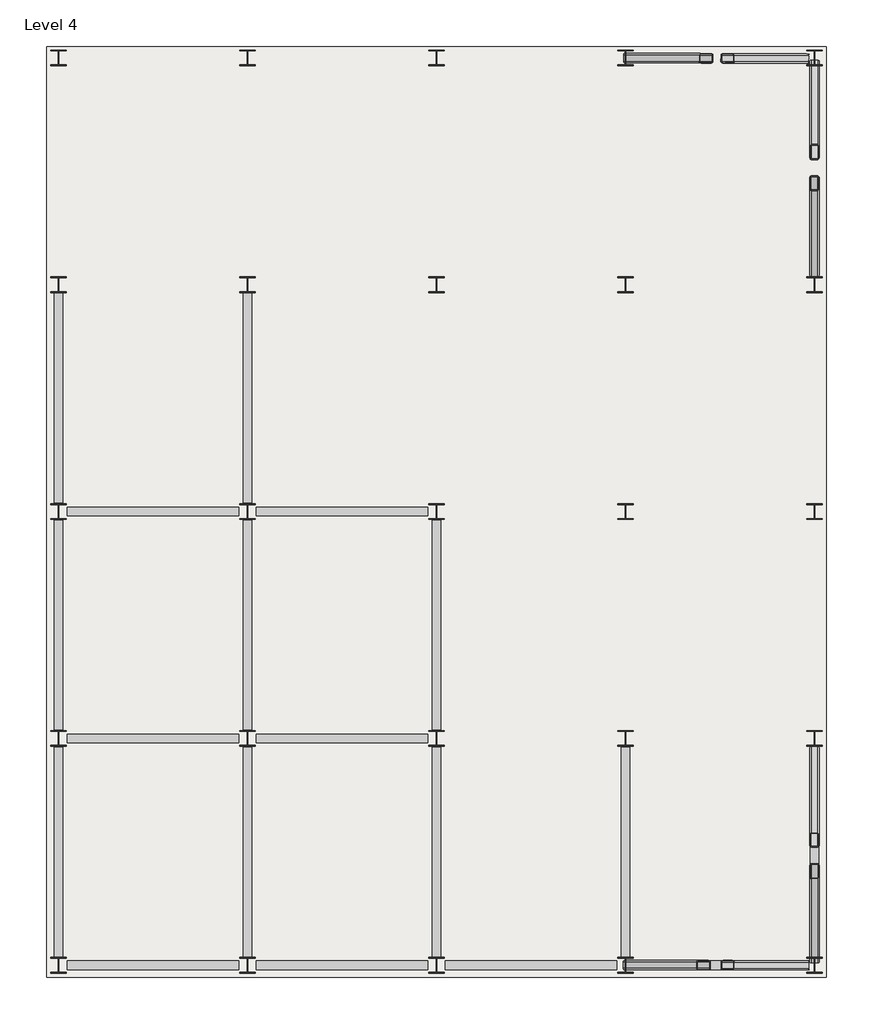
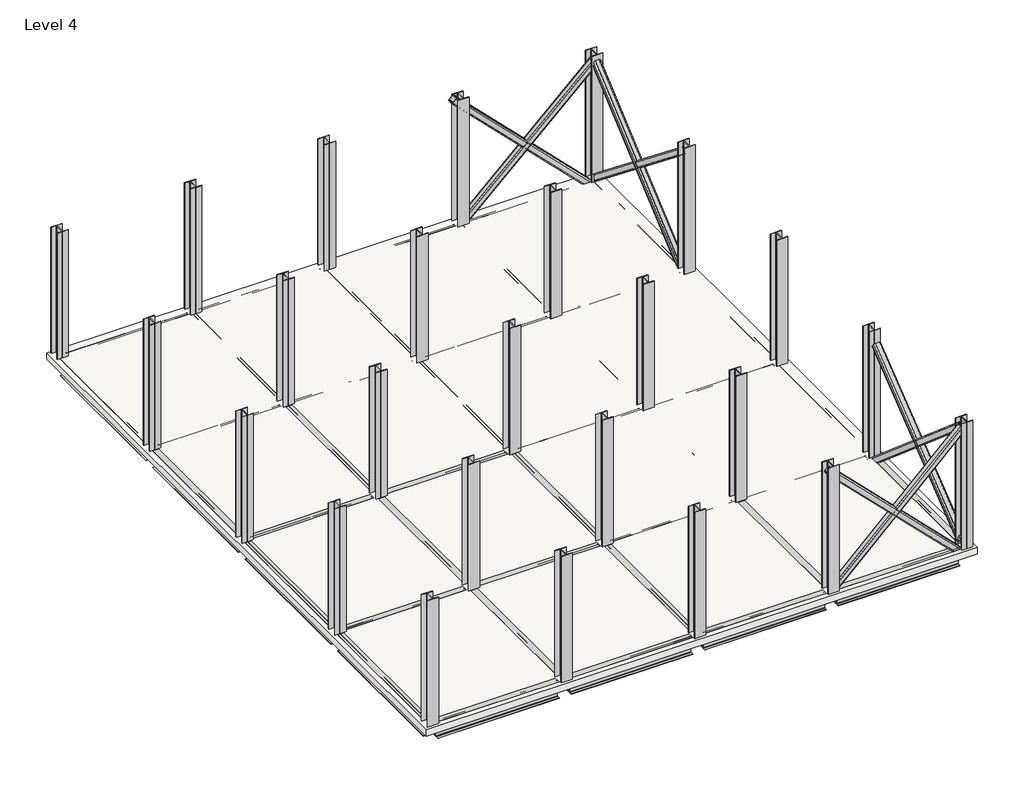
# One storey: 40 beams, 25 columns, 8 members, 1 slab.
"""IFC4 building model written with IfcOpenShell, lengths in millimetres."""

from ifc_helpers import new_model, si_unit, frame, origin, place, context, project, spatial, polyline, outline, extrude, transform, mapped, element, save
from components import w_shapes_w16x26_71b85d0e, w_shapes_w16x26_5730d789, w_shapes_column_w10x49_8035b166, hss_square_hss6x6x1_2_008024fe, hss_square_hss6x6x1_2_7c43692b, hss_square_hss6x6x1_2_5f011b37, hss_square_hss6x6x1_2_b9926e2d, hss_square_hss6x6x1_2_e6555cf9, hss_square_hss6x6x1_2_f7a49a43, hss_square_hss6x6x1_2_10b7330d, hss_square_hss6x6x1_2_f3b36863

model = new_model("IFC4")

# Units and contexts
model_context = context("Model", 3, world=origin())
ifc_project = project(units=[si_unit("LENGTHUNIT", "METRE", prefix="MILLI")], contexts=[model_context])

# Site, building, storey
site = spatial("IfcSite", under=ifc_project)
building = spatial("IfcBuilding", under=site)
storey = spatial("IfcBuildingStorey", under=building, Name="Level 4", Elevation=9144.0)

# Beams
placement = place(None, origin())
w_shapes_w16x26_shape = w_shapes_w16x26_71b85d0e(model_context)
element("IfcBeam", 1, ObjectType="W Shapes : W16X26", at=placement, inside=storey, context=model_context, shape_type="MappedRepresentation", body=[
    mapped(w_shapes_w16x26_shape, transform((-5883.5186598, -2213.7239423, 8944.61), x_axis=(1.0, 0.0, 0.0), y_axis=(0.0, 1.0, 0.0), z_axis=(0.0, 0.0, 1.0))),
])
element("IfcBeam", 2, ObjectType="W Shapes : W16X26", at=placement, inside=storey, context=model_context, shape_type="MappedRepresentation", body=[
    mapped(w_shapes_w16x26_shape, transform((-2835.5186598, -2213.7239423, 8944.61), x_axis=(1.0, 0.0, 0.0), y_axis=(0.0, 1.0, 0.0), z_axis=(0.0, 0.0, 1.0))),
])
element("IfcBeam", 3, ObjectType="W Shapes : W16X26", at=placement, inside=storey, context=model_context, shape_type="MappedRepresentation", body=[
    mapped(w_shapes_w16x26_shape, transform((212.4813402, -2213.7239423, 8944.61), x_axis=(1.0, 0.0, 0.0), y_axis=(0.0, 1.0, 0.0), z_axis=(0.0, 0.0, 1.0))),
])
element("IfcBeam", 4, ObjectType="W Shapes : W16X26", at=placement, inside=storey, context=model_context, shape_type="MappedRepresentation", body=[
    mapped(w_shapes_w16x26_shape, transform((3260.4813402, -2213.7239423, 8944.61), x_axis=(1.0, 0.0, 0.0), y_axis=(0.0, 1.0, 0.0), z_axis=(0.0, 0.0, 1.0))),
])
element("IfcBeam", 5, ObjectType="W Shapes : W16X26", at=placement, inside=storey, context=model_context, shape_type="MappedRepresentation", body=[
    mapped(w_shapes_w16x26_shape, transform((-5883.5186598, 1443.8760577, 8944.61), x_axis=(1.0, 0.0, 0.0), y_axis=(0.0, 1.0, 0.0), z_axis=(0.0, 0.0, 1.0))),
])
element("IfcBeam", 6, ObjectType="W Shapes : W16X26", at=placement, inside=storey, context=model_context, shape_type="MappedRepresentation", body=[
    mapped(w_shapes_w16x26_shape, transform((-2835.5186598, 1443.8760577, 8944.61), x_axis=(1.0, 0.0, 0.0), y_axis=(0.0, 1.0, 0.0), z_axis=(0.0, 0.0, 1.0))),
])
element("IfcBeam", 7, ObjectType="W Shapes : W16X26", at=placement, inside=storey, context=model_context, shape_type="MappedRepresentation", body=[
    mapped(w_shapes_w16x26_shape, transform((212.4813402, 1443.8760577, 8944.61), x_axis=(1.0, 0.0, 0.0), y_axis=(0.0, 1.0, 0.0), z_axis=(0.0, 0.0, 1.0))),
])
element("IfcBeam", 8, ObjectType="W Shapes : W16X26", at=placement, inside=storey, context=model_context, shape_type="MappedRepresentation", body=[
    mapped(w_shapes_w16x26_shape, transform((3260.4813402, 1443.8760577, 8944.61), x_axis=(1.0, 0.0, 0.0), y_axis=(0.0, 1.0, 0.0), z_axis=(0.0, 0.0, 1.0))),
])
element("IfcBeam", 9, ObjectType="W Shapes : W16X26", at=placement, inside=storey, context=model_context, shape_type="MappedRepresentation", body=[
    mapped(w_shapes_w16x26_shape, transform((-5883.5186598, 5101.4760577, 8944.61), x_axis=(1.0, 0.0, 0.0), y_axis=(0.0, 1.0, 0.0), z_axis=(0.0, 0.0, 1.0))),
])
element("IfcBeam", 10, ObjectType="W Shapes : W16X26", at=placement, inside=storey, context=model_context, shape_type="MappedRepresentation", body=[
    mapped(w_shapes_w16x26_shape, transform((-2835.5186598, 5101.4760577, 8944.61), x_axis=(1.0, 0.0, 0.0), y_axis=(0.0, 1.0, 0.0), z_axis=(0.0, 0.0, 1.0))),
])
element("IfcBeam", 11, ObjectType="W Shapes : W16X26", at=placement, inside=storey, context=model_context, shape_type="MappedRepresentation", body=[
    mapped(w_shapes_w16x26_shape, transform((212.4813402, 5101.4760577, 8944.61), x_axis=(1.0, 0.0, 0.0), y_axis=(0.0, 1.0, 0.0), z_axis=(0.0, 0.0, 1.0))),
])
element("IfcBeam", 12, ObjectType="W Shapes : W16X26", at=placement, inside=storey, context=model_context, shape_type="MappedRepresentation", body=[
    mapped(w_shapes_w16x26_shape, transform((3260.4813402, 5101.4760577, 8944.61), x_axis=(1.0, 0.0, 0.0), y_axis=(0.0, 1.0, 0.0), z_axis=(0.0, 0.0, 1.0))),
])
element("IfcBeam", 13, ObjectType="W Shapes : W16X26", at=placement, inside=storey, context=model_context, shape_type="MappedRepresentation", body=[
    mapped(w_shapes_w16x26_shape, transform((-5883.5186598, 8759.0760577, 8944.61), x_axis=(1.0, 0.0, 0.0), y_axis=(0.0, 1.0, 0.0), z_axis=(0.0, 0.0, 1.0))),
])
element("IfcBeam", 14, ObjectType="W Shapes : W16X26", at=placement, inside=storey, context=model_context, shape_type="MappedRepresentation", body=[
    mapped(w_shapes_w16x26_shape, transform((-2835.5186598, 8759.0760577, 8944.61), x_axis=(1.0, 0.0, 0.0), y_axis=(0.0, 1.0, 0.0), z_axis=(0.0, 0.0, 1.0))),
])
element("IfcBeam", 15, ObjectType="W Shapes : W16X26", at=placement, inside=storey, context=model_context, shape_type="MappedRepresentation", body=[
    mapped(w_shapes_w16x26_shape, transform((212.4813402, 8759.0760577, 8944.61), x_axis=(1.0, 0.0, 0.0), y_axis=(0.0, 1.0, 0.0), z_axis=(0.0, 0.0, 1.0))),
])
element("IfcBeam", 16, ObjectType="W Shapes : W16X26", at=placement, inside=storey, context=model_context, shape_type="MappedRepresentation", body=[
    mapped(w_shapes_w16x26_shape, transform((3260.4813402, 8759.0760577, 8944.61), x_axis=(1.0, 0.0, 0.0), y_axis=(0.0, 1.0, 0.0), z_axis=(0.0, 0.0, 1.0))),
])
element("IfcBeam", 17, ObjectType="W Shapes : W16X26", at=placement, inside=storey, context=model_context, shape_type="MappedRepresentation", body=[
    mapped(w_shapes_w16x26_shape, transform((-5883.5186598, 12416.6760577, 8944.61), x_axis=(1.0, 0.0, 0.0), y_axis=(0.0, 1.0, 0.0), z_axis=(0.0, 0.0, 1.0))),
])
element("IfcBeam", 18, ObjectType="W Shapes : W16X26", at=placement, inside=storey, context=model_context, shape_type="MappedRepresentation", body=[
    mapped(w_shapes_w16x26_shape, transform((-2835.5186598, 12416.6760577, 8944.61), x_axis=(1.0, 0.0, 0.0), y_axis=(0.0, 1.0, 0.0), z_axis=(0.0, 0.0, 1.0))),
])
element("IfcBeam", 19, ObjectType="W Shapes : W16X26", at=placement, inside=storey, context=model_context, shape_type="MappedRepresentation", body=[
    mapped(w_shapes_w16x26_shape, transform((212.4813402, 12416.6760577, 8944.61), x_axis=(1.0, 0.0, 0.0), y_axis=(0.0, 1.0, 0.0), z_axis=(0.0, 0.0, 1.0))),
])
element("IfcBeam", 20, ObjectType="W Shapes : W16X26", at=placement, inside=storey, context=model_context, shape_type="MappedRepresentation", body=[
    mapped(w_shapes_w16x26_shape, transform((3260.4813402, 12416.6760577, 8944.61), x_axis=(1.0, 0.0, 0.0), y_axis=(0.0, 1.0, 0.0), z_axis=(0.0, 0.0, 1.0))),
])
w_shapes_w16x26_2_shape = w_shapes_w16x26_5730d789(model_context)
element("IfcBeam", 21, ObjectType="W Shapes : W16X26", at=placement, inside=storey, context=model_context, shape_type="MappedRepresentation", body=[
    mapped(w_shapes_w16x26_2_shape, transform((4784.4813402, 10587.8760577, 8944.61), x_axis=(0.0, -1.0, 0.0), y_axis=(1.0, 0.0, 0.0), z_axis=(0.0, 0.0, 1.0))),
])
element("IfcBeam", 22, ObjectType="W Shapes : W16X26", at=placement, inside=storey, context=model_context, shape_type="MappedRepresentation", body=[
    mapped(w_shapes_w16x26_2_shape, transform((4784.4813402, 6930.2760577, 8944.61), x_axis=(0.0, -1.0, 0.0), y_axis=(1.0, 0.0, 0.0), z_axis=(0.0, 0.0, 1.0))),
])
element("IfcBeam", 23, ObjectType="W Shapes : W16X26", at=placement, inside=storey, context=model_context, shape_type="MappedRepresentation", body=[
    mapped(w_shapes_w16x26_2_shape, transform((4784.4813402, 3272.6760577, 8944.61), x_axis=(0.0, -1.0, 0.0), y_axis=(1.0, 0.0, 0.0), z_axis=(0.0, 0.0, 1.0))),
])
element("IfcBeam", 24, ObjectType="W Shapes : W16X26", at=placement, inside=storey, context=model_context, shape_type="MappedRepresentation", body=[
    mapped(w_shapes_w16x26_2_shape, transform((4784.4813402, -384.9239423, 8944.61), x_axis=(0.0, -1.0, 0.0), y_axis=(1.0, 0.0, 0.0), z_axis=(0.0, 0.0, 1.0))),
])
element("IfcBeam", 25, ObjectType="W Shapes : W16X26", at=placement, inside=storey, context=model_context, shape_type="MappedRepresentation", body=[
    mapped(w_shapes_w16x26_2_shape, transform((1736.4813402, 10587.8760577, 8944.61), x_axis=(0.0, -1.0, 0.0), y_axis=(1.0, 0.0, 0.0), z_axis=(0.0, 0.0, 1.0))),
])
element("IfcBeam", 26, ObjectType="W Shapes : W16X26", at=placement, inside=storey, context=model_context, shape_type="MappedRepresentation", body=[
    mapped(w_shapes_w16x26_2_shape, transform((1736.4813402, 6930.2760577, 8944.61), x_axis=(0.0, -1.0, 0.0), y_axis=(1.0, 0.0, 0.0), z_axis=(0.0, 0.0, 1.0))),
])
element("IfcBeam", 27, ObjectType="W Shapes : W16X26", at=placement, inside=storey, context=model_context, shape_type="MappedRepresentation", body=[
    mapped(w_shapes_w16x26_2_shape, transform((1736.4813402, 3272.6760577, 8944.61), x_axis=(0.0, -1.0, 0.0), y_axis=(1.0, 0.0, 0.0), z_axis=(0.0, 0.0, 1.0))),
])
element("IfcBeam", 28, ObjectType="W Shapes : W16X26", at=placement, inside=storey, context=model_context, shape_type="MappedRepresentation", body=[
    mapped(w_shapes_w16x26_2_shape, transform((1736.4813402, -384.9239423, 8944.61), x_axis=(0.0, -1.0, 0.0), y_axis=(1.0, 0.0, 0.0), z_axis=(0.0, 0.0, 1.0))),
])
element("IfcBeam", 29, ObjectType="W Shapes : W16X26", at=placement, inside=storey, context=model_context, shape_type="MappedRepresentation", body=[
    mapped(w_shapes_w16x26_2_shape, transform((-1311.5186598, 10587.8760577, 8944.61), x_axis=(0.0, -1.0, 0.0), y_axis=(1.0, 0.0, 0.0), z_axis=(0.0, 0.0, 1.0))),
])
element("IfcBeam", 30, ObjectType="W Shapes : W16X26", at=placement, inside=storey, context=model_context, shape_type="MappedRepresentation", body=[
    mapped(w_shapes_w16x26_2_shape, transform((-1311.5186598, 6930.2760577, 8944.61), x_axis=(0.0, -1.0, 0.0), y_axis=(1.0, 0.0, 0.0), z_axis=(0.0, 0.0, 1.0))),
])
element("IfcBeam", 31, ObjectType="W Shapes : W16X26", at=placement, inside=storey, context=model_context, shape_type="MappedRepresentation", body=[
    mapped(w_shapes_w16x26_2_shape, transform((-1311.5186598, 3272.6760577, 8944.61), x_axis=(0.0, -1.0, 0.0), y_axis=(1.0, 0.0, 0.0), z_axis=(0.0, 0.0, 1.0))),
])
element("IfcBeam", 32, ObjectType="W Shapes : W16X26", at=placement, inside=storey, context=model_context, shape_type="MappedRepresentation", body=[
    mapped(w_shapes_w16x26_2_shape, transform((-1311.5186598, -384.9239423, 8944.61), x_axis=(0.0, -1.0, 0.0), y_axis=(1.0, 0.0, 0.0), z_axis=(0.0, 0.0, 1.0))),
])
element("IfcBeam", 33, ObjectType="W Shapes : W16X26", at=placement, inside=storey, context=model_context, shape_type="MappedRepresentation", body=[
    mapped(w_shapes_w16x26_2_shape, transform((-4359.5186598, 10587.8760577, 8944.61), x_axis=(0.0, -1.0, 0.0), y_axis=(1.0, 0.0, 0.0), z_axis=(0.0, 0.0, 1.0))),
])
element("IfcBeam", 34, ObjectType="W Shapes : W16X26", at=placement, inside=storey, context=model_context, shape_type="MappedRepresentation", body=[
    mapped(w_shapes_w16x26_2_shape, transform((-4359.5186598, 6930.2760577, 8944.61), x_axis=(0.0, -1.0, 0.0), y_axis=(1.0, 0.0, 0.0), z_axis=(0.0, 0.0, 1.0))),
])
element("IfcBeam", 35, ObjectType="W Shapes : W16X26", at=placement, inside=storey, context=model_context, shape_type="MappedRepresentation", body=[
    mapped(w_shapes_w16x26_2_shape, transform((-4359.5186598, 3272.6760577, 8944.61), x_axis=(0.0, -1.0, 0.0), y_axis=(1.0, 0.0, 0.0), z_axis=(0.0, 0.0, 1.0))),
])
element("IfcBeam", 36, ObjectType="W Shapes : W16X26", at=placement, inside=storey, context=model_context, shape_type="MappedRepresentation", body=[
    mapped(w_shapes_w16x26_2_shape, transform((-4359.5186598, -384.9239423, 8944.61), x_axis=(0.0, -1.0, 0.0), y_axis=(1.0, 0.0, 0.0), z_axis=(0.0, 0.0, 1.0))),
])
element("IfcBeam", 37, ObjectType="W Shapes : W16X26", at=placement, inside=storey, context=model_context, shape_type="MappedRepresentation", body=[
    mapped(w_shapes_w16x26_2_shape, transform((-7407.5186598, 10587.8760577, 8944.61), x_axis=(0.0, -1.0, 0.0), y_axis=(1.0, 0.0, 0.0), z_axis=(0.0, 0.0, 1.0))),
])
element("IfcBeam", 38, ObjectType="W Shapes : W16X26", at=placement, inside=storey, context=model_context, shape_type="MappedRepresentation", body=[
    mapped(w_shapes_w16x26_2_shape, transform((-7407.5186598, 6930.2760577, 8944.61), x_axis=(0.0, -1.0, 0.0), y_axis=(1.0, 0.0, 0.0), z_axis=(0.0, 0.0, 1.0))),
])
element("IfcBeam", 39, ObjectType="W Shapes : W16X26", at=placement, inside=storey, context=model_context, shape_type="MappedRepresentation", body=[
    mapped(w_shapes_w16x26_2_shape, transform((-7407.5186598, 3272.6760577, 8944.61), x_axis=(0.0, -1.0, 0.0), y_axis=(1.0, 0.0, 0.0), z_axis=(0.0, 0.0, 1.0))),
])
element("IfcBeam", 40, ObjectType="W Shapes : W16X26", at=placement, inside=storey, context=model_context, shape_type="MappedRepresentation", body=[
    mapped(w_shapes_w16x26_2_shape, transform((-7407.5186598, -384.9239423, 8944.61), x_axis=(0.0, -1.0, 0.0), y_axis=(1.0, 0.0, 0.0), z_axis=(0.0, 0.0, 1.0))),
])

# Columns
w_shapes_column_w10x49_shape = w_shapes_column_w10x49_8035b166(model_context)
element("IfcColumn", 41, ObjectType="W Shapes-Column : W10X49", at=placement, inside=storey, context=model_context, shape_type="MappedRepresentation", body=[
    mapped(w_shapes_column_w10x49_shape, transform((4784.4813402, -2213.7239423, 0.0), x_axis=(1.0, 0.0, 0.0), y_axis=(0.0, 1.0, 0.0), z_axis=(0.0, 0.0, 1.0))),
])
element("IfcColumn", 42, ObjectType="W Shapes-Column : W10X49", at=placement, inside=storey, context=model_context, shape_type="MappedRepresentation", body=[
    mapped(w_shapes_column_w10x49_shape, transform((1736.4813402, -2213.7239423, 0.0), x_axis=(1.0, 0.0, 0.0), y_axis=(0.0, 1.0, 0.0), z_axis=(0.0, 0.0, 1.0))),
])
element("IfcColumn", 43, ObjectType="W Shapes-Column : W10X49", at=placement, inside=storey, context=model_context, shape_type="MappedRepresentation", body=[
    mapped(w_shapes_column_w10x49_shape, transform((-1311.5186598, -2213.7239423, 0.0), x_axis=(1.0, 0.0, 0.0), y_axis=(0.0, 1.0, 0.0), z_axis=(0.0, 0.0, 1.0))),
])
element("IfcColumn", 44, ObjectType="W Shapes-Column : W10X49", at=placement, inside=storey, context=model_context, shape_type="MappedRepresentation", body=[
    mapped(w_shapes_column_w10x49_shape, transform((-4359.5186598, -2213.7239423, 0.0), x_axis=(1.0, 0.0, 0.0), y_axis=(0.0, 1.0, 0.0), z_axis=(0.0, 0.0, 1.0))),
])
element("IfcColumn", 45, ObjectType="W Shapes-Column : W10X49", at=placement, inside=storey, context=model_context, shape_type="MappedRepresentation", body=[
    mapped(w_shapes_column_w10x49_shape, transform((-7407.5186598, -2213.7239423, 0.0), x_axis=(1.0, 0.0, 0.0), y_axis=(0.0, 1.0, 0.0), z_axis=(0.0, 0.0, 1.0))),
])
element("IfcColumn", 46, ObjectType="W Shapes-Column : W10X49", at=placement, inside=storey, context=model_context, shape_type="MappedRepresentation", body=[
    mapped(w_shapes_column_w10x49_shape, transform((4784.4813402, 1443.8760577, 0.0), x_axis=(1.0, 0.0, 0.0), y_axis=(0.0, 1.0, 0.0), z_axis=(0.0, 0.0, 1.0))),
])
element("IfcColumn", 47, ObjectType="W Shapes-Column : W10X49", at=placement, inside=storey, context=model_context, shape_type="MappedRepresentation", body=[
    mapped(w_shapes_column_w10x49_shape, transform((4784.4813402, 5101.4760577, 0.0), x_axis=(1.0, 0.0, 0.0), y_axis=(0.0, 1.0, 0.0), z_axis=(0.0, 0.0, 1.0))),
])
element("IfcColumn", 48, ObjectType="W Shapes-Column : W10X49", at=placement, inside=storey, context=model_context, shape_type="MappedRepresentation", body=[
    mapped(w_shapes_column_w10x49_shape, transform((4784.4813402, 8759.0760577, 0.0), x_axis=(1.0, 0.0, 0.0), y_axis=(0.0, 1.0, 0.0), z_axis=(0.0, 0.0, 1.0))),
])
element("IfcColumn", 49, ObjectType="W Shapes-Column : W10X49", at=placement, inside=storey, context=model_context, shape_type="MappedRepresentation", body=[
    mapped(w_shapes_column_w10x49_shape, transform((4784.4813402, 12416.6760577, 0.0), x_axis=(1.0, 0.0, 0.0), y_axis=(0.0, 1.0, 0.0), z_axis=(0.0, 0.0, 1.0))),
])
element("IfcColumn", 50, ObjectType="W Shapes-Column : W10X49", at=placement, inside=storey, context=model_context, shape_type="MappedRepresentation", body=[
    mapped(w_shapes_column_w10x49_shape, transform((1736.4813402, 1443.8760577, 0.0), x_axis=(1.0, 0.0, 0.0), y_axis=(0.0, 1.0, 0.0), z_axis=(0.0, 0.0, 1.0))),
])
element("IfcColumn", 51, ObjectType="W Shapes-Column : W10X49", at=placement, inside=storey, context=model_context, shape_type="MappedRepresentation", body=[
    mapped(w_shapes_column_w10x49_shape, transform((-1311.5186598, 1443.8760577, 0.0), x_axis=(1.0, 0.0, 0.0), y_axis=(0.0, 1.0, 0.0), z_axis=(0.0, 0.0, 1.0))),
])
element("IfcColumn", 52, ObjectType="W Shapes-Column : W10X49", at=placement, inside=storey, context=model_context, shape_type="MappedRepresentation", body=[
    mapped(w_shapes_column_w10x49_shape, transform((-4359.5186598, 1443.8760577, 0.0), x_axis=(1.0, 0.0, 0.0), y_axis=(0.0, 1.0, 0.0), z_axis=(0.0, 0.0, 1.0))),
])
element("IfcColumn", 53, ObjectType="W Shapes-Column : W10X49", at=placement, inside=storey, context=model_context, shape_type="MappedRepresentation", body=[
    mapped(w_shapes_column_w10x49_shape, transform((-7407.5186598, 1443.8760577, 0.0), x_axis=(1.0, 0.0, 0.0), y_axis=(0.0, 1.0, 0.0), z_axis=(0.0, 0.0, 1.0))),
])
element("IfcColumn", 54, ObjectType="W Shapes-Column : W10X49", at=placement, inside=storey, context=model_context, shape_type="MappedRepresentation", body=[
    mapped(w_shapes_column_w10x49_shape, transform((1736.4813402, 5101.4760577, 0.0), x_axis=(1.0, 0.0, 0.0), y_axis=(0.0, 1.0, 0.0), z_axis=(0.0, 0.0, 1.0))),
])
element("IfcColumn", 55, ObjectType="W Shapes-Column : W10X49", at=placement, inside=storey, context=model_context, shape_type="MappedRepresentation", body=[
    mapped(w_shapes_column_w10x49_shape, transform((-1311.5186598, 5101.4760577, 0.0), x_axis=(1.0, 0.0, 0.0), y_axis=(0.0, 1.0, 0.0), z_axis=(0.0, 0.0, 1.0))),
])
element("IfcColumn", 56, ObjectType="W Shapes-Column : W10X49", at=placement, inside=storey, context=model_context, shape_type="MappedRepresentation", body=[
    mapped(w_shapes_column_w10x49_shape, transform((-4359.5186598, 5101.4760577, 0.0), x_axis=(1.0, 0.0, 0.0), y_axis=(0.0, 1.0, 0.0), z_axis=(0.0, 0.0, 1.0))),
])
element("IfcColumn", 57, ObjectType="W Shapes-Column : W10X49", at=placement, inside=storey, context=model_context, shape_type="MappedRepresentation", body=[
    mapped(w_shapes_column_w10x49_shape, transform((-7407.5186598, 5101.4760577, 0.0), x_axis=(1.0, 0.0, 0.0), y_axis=(0.0, 1.0, 0.0), z_axis=(0.0, 0.0, 1.0))),
])
element("IfcColumn", 58, ObjectType="W Shapes-Column : W10X49", at=placement, inside=storey, context=model_context, shape_type="MappedRepresentation", body=[
    mapped(w_shapes_column_w10x49_shape, transform((1736.4813402, 8759.0760577, 0.0), x_axis=(1.0, 0.0, 0.0), y_axis=(0.0, 1.0, 0.0), z_axis=(0.0, 0.0, 1.0))),
])
element("IfcColumn", 59, ObjectType="W Shapes-Column : W10X49", at=placement, inside=storey, context=model_context, shape_type="MappedRepresentation", body=[
    mapped(w_shapes_column_w10x49_shape, transform((-1311.5186598, 8759.0760577, 0.0), x_axis=(1.0, 0.0, 0.0), y_axis=(0.0, 1.0, 0.0), z_axis=(0.0, 0.0, 1.0))),
])
element("IfcColumn", 60, ObjectType="W Shapes-Column : W10X49", at=placement, inside=storey, context=model_context, shape_type="MappedRepresentation", body=[
    mapped(w_shapes_column_w10x49_shape, transform((-4359.5186598, 8759.0760577, 0.0), x_axis=(1.0, 0.0, 0.0), y_axis=(0.0, 1.0, 0.0), z_axis=(0.0, 0.0, 1.0))),
])
element("IfcColumn", 61, ObjectType="W Shapes-Column : W10X49", at=placement, inside=storey, context=model_context, shape_type="MappedRepresentation", body=[
    mapped(w_shapes_column_w10x49_shape, transform((-7407.5186598, 8759.0760577, 0.0), x_axis=(1.0, 0.0, 0.0), y_axis=(0.0, 1.0, 0.0), z_axis=(0.0, 0.0, 1.0))),
])
element("IfcColumn", 62, ObjectType="W Shapes-Column : W10X49", at=placement, inside=storey, context=model_context, shape_type="MappedRepresentation", body=[
    mapped(w_shapes_column_w10x49_shape, transform((1736.4813402, 12416.6760577, 0.0), x_axis=(1.0, 0.0, 0.0), y_axis=(0.0, 1.0, 0.0), z_axis=(0.0, 0.0, 1.0))),
])
element("IfcColumn", 63, ObjectType="W Shapes-Column : W10X49", at=placement, inside=storey, context=model_context, shape_type="MappedRepresentation", body=[
    mapped(w_shapes_column_w10x49_shape, transform((-1311.5186598, 12416.6760577, 0.0), x_axis=(1.0, 0.0, 0.0), y_axis=(0.0, 1.0, 0.0), z_axis=(0.0, 0.0, 1.0))),
])
element("IfcColumn", 64, ObjectType="W Shapes-Column : W10X49", at=placement, inside=storey, context=model_context, shape_type="MappedRepresentation", body=[
    mapped(w_shapes_column_w10x49_shape, transform((-4359.5186598, 12416.6760577, 0.0), x_axis=(1.0, 0.0, 0.0), y_axis=(0.0, 1.0, 0.0), z_axis=(0.0, 0.0, 1.0))),
])
element("IfcColumn", 65, ObjectType="W Shapes-Column : W10X49", at=placement, inside=storey, context=model_context, shape_type="MappedRepresentation", body=[
    mapped(w_shapes_column_w10x49_shape, transform((-7407.5186598, 12416.6760577, 0.0), x_axis=(1.0, 0.0, 0.0), y_axis=(0.0, 1.0, 0.0), z_axis=(0.0, 0.0, 1.0))),
])

# Members
hss_square_hss6x6x1_2_shape = hss_square_hss6x6x1_2_008024fe(model_context)
element("IfcMember", 66, ObjectType="HSS Square : HSS6X6X1/2", at=placement, inside=storey, context=model_context, shape_type="MappedRepresentation", body=[
    mapped(hss_square_hss6x6x1_2_shape, transform((4784.4813402, 10587.8760577, 10591.8), x_axis=(0.0, 0.7840458244617616, -0.6207029443655613), y_axis=(-1.0000000000000002, 0.0, 0.0), z_axis=(0.0, 0.6207029443655613, 0.7840458244617616))),
])
hss_square_hss6x6x1_2_2_shape = hss_square_hss6x6x1_2_7c43692b(model_context)
element("IfcMember", 67, ObjectType="HSS Square : HSS6X6X1/2", at=placement, inside=storey, context=model_context, shape_type="MappedRepresentation", body=[
    mapped(hss_square_hss6x6x1_2_2_shape, transform((4784.4813402, 10587.8760577, 10508.1631022), x_axis=(0.0, -0.7600753460328191, -0.6498349547024158), y_axis=(1.0000000000000002, 0.0, 0.0), z_axis=(0.0, -0.6498349547024158, 0.7600753460328191))),
])
hss_square_hss6x6x1_2_3_shape = hss_square_hss6x6x1_2_5f011b37(model_context)
element("IfcMember", 68, ObjectType="HSS Square : HSS6X6X1/2", at=placement, inside=storey, context=model_context, shape_type="MappedRepresentation", body=[
    mapped(hss_square_hss6x6x1_2_3_shape, transform((4784.4813402, -384.9239423, 10508.1631022), x_axis=(0.0, 0.7600753460328191, -0.6498349547024158), y_axis=(-1.0000000000000002, 0.0, 0.0), z_axis=(0.0, 0.6498349547024158, 0.7600753460328191))),
])
hss_square_hss6x6x1_2_4_shape = hss_square_hss6x6x1_2_b9926e2d(model_context)
element("IfcMember", 69, ObjectType="HSS Square : HSS6X6X1/2", at=placement, inside=storey, context=model_context, shape_type="MappedRepresentation", body=[
    mapped(hss_square_hss6x6x1_2_4_shape, transform((4784.4813402, -384.9239423, 10591.8), x_axis=(0.0, -0.7840458244617616, -0.6207029443655613), y_axis=(1.0000000000000002, 0.0, 0.0), z_axis=(0.0, -0.6207029443655613, 0.7840458244617616))),
])
hss_square_hss6x6x1_2_5_shape = hss_square_hss6x6x1_2_e6555cf9(model_context)
element("IfcMember", 70, ObjectType="HSS Square : HSS6X6X1/2", at=placement, inside=storey, context=model_context, shape_type="MappedRepresentation", body=[
    mapped(hss_square_hss6x6x1_2_5_shape, transform((3168.0352384, -2213.7239423, 10509.8521986), x_axis=(-0.718393447364439, 0.0, -0.6956370136672122), y_axis=(0.0, -1.0000000000000002, 0.0), z_axis=(-0.6956370136672122, 0.0, 0.718393447364439))),
])
hss_square_hss6x6x1_2_6_shape = hss_square_hss6x6x1_2_f7a49a43(model_context)
element("IfcMember", 71, ObjectType="HSS Square : HSS6X6X1/2", at=placement, inside=storey, context=model_context, shape_type="MappedRepresentation", body=[
    mapped(hss_square_hss6x6x1_2_6_shape, transform((3260.4813402, -2213.7239423, 10468.61), x_axis=(0.7071067811865474, 0.0, -0.7071067811865478), y_axis=(0.0, 1.0000000000000002, 0.0), z_axis=(0.7071067811865478, 0.0, 0.7071067811865474))),
])
hss_square_hss6x6x1_2_7_shape = hss_square_hss6x6x1_2_10b7330d(model_context)
element("IfcMember", 72, ObjectType="HSS Square : HSS6X6X1/2", at=placement, inside=storey, context=model_context, shape_type="MappedRepresentation", body=[
    mapped(hss_square_hss6x6x1_2_7_shape, transform((3168.0352384, 12409.9819642, 10468.61), x_axis=(-0.7276035720332943, 0.003013182054487384, -0.6859912264003801), y_axis=(-0.004141205915939178, -0.9999914251700173, 0.0), z_axis=(-0.685985344142244, 0.0028408309250507737, 0.7276098111637189))),
])
hss_square_hss6x6x1_2_8_shape = hss_square_hss6x6x1_2_f3b36863(model_context)
element("IfcMember", 73, ObjectType="HSS Square : HSS6X6X1/2", at=placement, inside=storey, context=model_context, shape_type="MappedRepresentation", body=[
    mapped(hss_square_hss6x6x1_2_8_shape, transform((3260.4813402, 12409.9819642, 10468.61), x_axis=(0.7071033705496139, -0.003105916088734984, -0.7071033705496145), y_axis=(0.004392407470180803, 0.9999903533317791, 0.0), z_axis=(0.7070965493580007, -0.003105886126991346, 0.70711019180703))),
])

# Slab
element("IfcSlab", 74, ObjectType="6\" Foundation Slab", at=placement, inside=storey, context=model_context, shape_type="SweptSolid", body=[
    extrude(outline(polyline([(4974.3230176, 12600.4819642), (4974.3230176, -2410.9180358), (-7598.6769824, -2410.9180358), (-7598.6769824, 12600.4819642), (4974.3230176, 12600.4819642)])), frame((0.0, 0.0, 8991.6), z_axis=(0.0, 0.0, 1.0), x_axis=(1.0, 0.0, 0.0)), (0.0, 0.0, 1.0), 152.4),
])

save(model, "model.ifc")

# Revit data of these elements
# Type "W Shapes : W16X26"
#   Section Name Key = "W16x26"
#   Assembly Code = "B10"
#   Width = 5.500"
#   Web Thickness = 0.250"
#   Web Fillet = 0.402"
#   Warping Constant = 565.00 in⁶
#   Torsional Moment of Inertia = 0.262 in⁴
#   Section Area = 7.68 in²
#   Plastic Modulus weak axis = 5.48 in³
#   Plastic Modulus strong axis = 44.20 in³
#   Perimeter = 52.20 ft²/ft
#   Nominal Weight = 26.00 lbf/ft
#   Moment of Inertia weak axis = 9.59 in⁴
#   Moment of Inertia strong axis = 301.00 in⁴
#   Height = 15.700"
#   Flange Thickness = 0.345"
#   Elastic Modulus weak axis = 3.49 in³
#   Elastic Modulus strong axis = 38.40 in³
#   Centroid Vertical = 7.850"
#   Centroid Horizontal = 2.750"
#   Bolt Spacing = 0' - 3 1/2"
#   Length [instance default] = 5' - 0"
#   Structural Material [instance default] = Steel ASTM A992
#   Principal Axes Angle = 0
# Type "W Shapes-Column : W10X49"
#   Section Name Key = "W10x49"
#   Assembly Code = "B10"
#   Width = 10.000"
#   Web Thickness = 0.340"
#   Web Fillet = 0.500"
#   Warping Constant = 2070.00 in⁶
#   Torsional Moment of Inertia = 1.39 in⁴
#   Section Area = 14.40 in²
#   Plastic Modulus weak axis = 28.30 in³
#   Plastic Modulus strong axis = 60.40 in³
#   Perimeter = 58.50 ft²/ft
#   Nominal Weight = 49.00 lbf/ft
#   Moment of Inertia weak axis = 93.40 in⁴
#   Moment of Inertia strong axis = 272.00 in⁴
#   Height = 10.000"
#   Flange Thickness = 0.560"
#   Elastic Modulus weak axis = 18.70 in³
#   Elastic Modulus strong axis = 54.60 in³
#   Centroid Vertical = 5.000"
#   Centroid Horizontal = 5.000"
#   Bolt Spacing = 0' - 5 1/2"
#   Structural Material [instance default] = Steel ASTM A992
#   Principal Axes Angle = 0
# Type "HSS Square : HSS6X6X1/2"
#   Section Name Key = "HSS 6X6X1/2"
#   Assembly Code = "B10"
#   Width = 6.000"
#   Wall Nominal Thickness = 0.500"
#   Wall Design Thickness = 0.465"
#   Torsional Moment of Inertia = 81.10 in⁴
#   Torsional Modulus = 28.10 in³
#   Section Area = 9.74 in²
#   Plastic Modulus weak axis = 19.80 in³
#   Plastic Modulus strong axis = 19.80 in³
#   Outer Fillet = 1.000"
#   Nominal Weight = 35.24 lbf/ft
#   Moment of Inertia weak axis = 48.30 in⁴
#   Moment of Inertia strong axis = 48.30 in⁴
#   Inner Fillet = 0.500"
#   Height = 6.000"
#   Elastic Modulus weak axis = 16.10 in³
#   Elastic Modulus strong axis = 16.10 in³
#   Centroid Vertical = 3.000"
#   Centroid Horizontal = 3.000"
#   Length [instance default] = 5' - 0"
#   Structural Material [instance default] = Steel ASTM A500, Grade B, Rectangular and Square
#   Principal Axes Angle = 0
# Type "6\" Foundation Slab"
#   Layers, outside or top first: 0' - 6" "Concrete, Cast-in-Place gray" (function 1)
# Elements 1, 2, 3, 4, 5, 6, 7, 8, 9, 10, 11, 12, 13, 14, 15, 16, 17, 18, 19, 20, 21, 22, 23, 24, 25, 26, 27, 28, 29, 30, 31, 32, 33, 34, 35, 36, 37, 38, 39, 40 (IfcBeam, "W Shapes : W16X26")
#   Comments = ""
#   Structural Material = Steel ASTM A992
#   Phase Created = New Construction
#   Materials on its faces: "Steel ASTM A992"
# Elements 41, 42, 43, 44, 45, 46, 47, 48, 49, 50, 51, 52, 53, 54, 55, 56, 57, 58, 59, 60, 61, 62, 63, 64, 65 (IfcColumn, "W Shapes-Column : W10X49")
#   Structural Material = Steel ASTM A992
#   Phase Created = New Construction
#   Materials on its faces: "Steel ASTM A992"
# Elements 66, 67, 68, 69, 70, 71, 72, 73 (IfcMember, "HSS Square : HSS6X6X1/2")
#   Comments = ""
#   Structural Material = Steel ASTM A992
#   Phase Created = New Construction
#   Materials on its faces: "Steel ASTM A992"
# Element 74 (IfcSlab, "6\" Foundation Slab")
#   Height Offset From Level = 0' - 0"
#   built-in parameter 1001954 = 1
#   Phase Created = New Construction
#   Materials on its faces: "Concrete, Cast-in-Place gray"
# Materials
#   "Steel ASTM A992": class "Metal", colour RGB 199 199 199, transparency 0, Description = "Structural steel 50ksi", Cost = 0
#   "Steel ASTM A500, Grade B, Rectangular and Square": class "Metal", colour RGB 199 199 199, transparency 0, Description = "Carbon steel", Cost = 0
#   "Concrete, Cast-in-Place gray": class "Concrete", colour RGB 192 192 192, transparency 0, Description = "Cast-in-place concrete", Cost = 0
